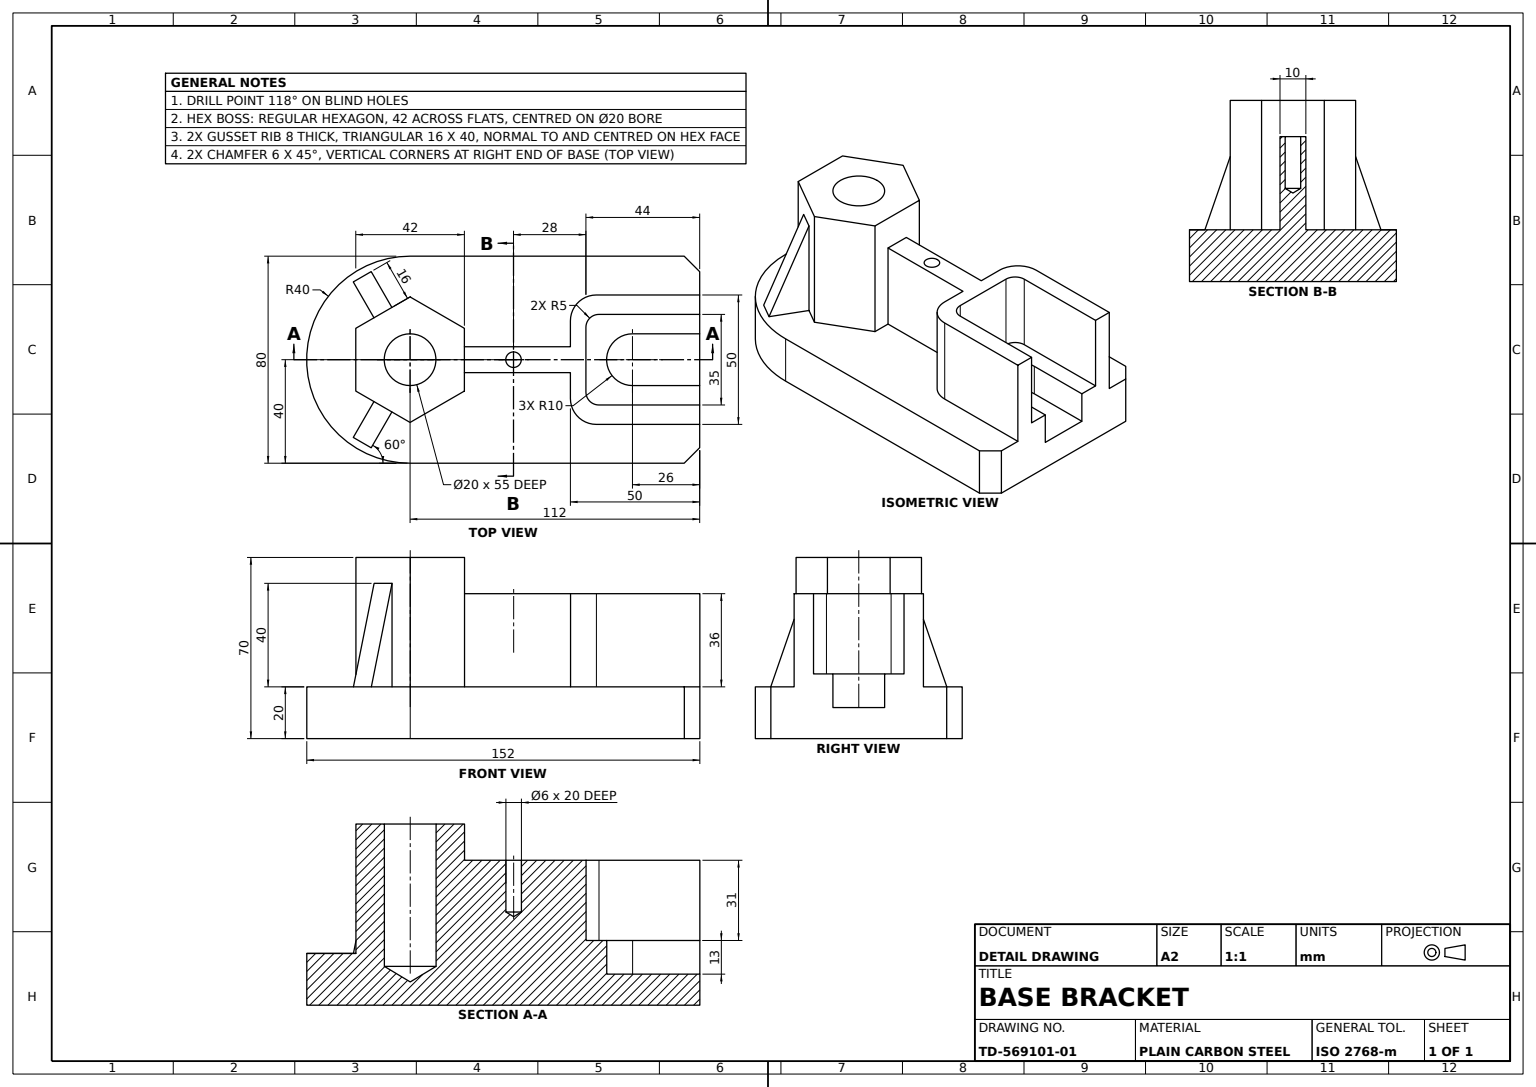
from build123d import *

# Parameters (mm, degrees)
BASE_PLATE_DEPTH        = 20
HEX_MOUNTING_BOSS_DEPTH = 50
GUSSET_RIB_1_SKETCH_W   = 8
GUSSET_RIB_1_SKETCH_H   = 40
GUSSET_RIB_1_DEPTH      = 16
RIB_1_TRIM_CUT_DEPTH    = 16
GUSSET_RIB_2_SKETCH_W   = 8
GUSSET_RIB_2_SKETCH_H   = 40
GUSSET_RIB_2_DEPTH      = 16
RIB_2_TRIM_CUT_DEPTH    = 16
BOSS_BORE_20_D          = 20
BOSS_BORE_20_DEPTH      = 55
BOSS_BORE_20_TIP        = 6.00860619
SHAFT_HOUSING_DEPTH     = 36
HOUSING_FILLET_R10_R    = 10
HOUSING_POCKET_DEPTH    = 31
HOUSING_SLOT_DEPTH      = 13
CROSS_HOLE_6_D          = 6
CROSS_HOLE_6_DEPTH      = 20
CROSS_HOLE_6_TIP        = 1.802581857


with BuildPart() as part:
    # Base Plate Sketch → Base Plate (new body)
    with BuildSketch(Plane(origin=(0, 0, 0), x_dir=(1, 0, 0), z_dir=(0, 1, 0))):
        with BuildLine():
            Line((0, 40), (106, 40))
            Line((106, 40), (112, 34))
            Line((112, 34), (112, -34))
            Line((112, -34), (106, -40))
            Line((106, -40), (0, -40))
            ThreePointArc((0, -40), (-40, 0), (0, 40))
        make_face()
    extrude(amount=BASE_PLATE_DEPTH)

    # Hex Boss Sketch → Hex Mounting Boss (add)
    with BuildSketch(Plane(origin=(0, 20, 0), x_dir=(1, 0, 0), z_dir=(0, 1, 0))):
        Polygon((0, 24.248711306), (-21, 12.124355653), (-21, -12.124355653), (0, -24.248711306), (21, -12.124355653), (21, 12.124355653), align=None)
    extrude(amount=HEX_MOUNTING_BOSS_DEPTH)

    # Gusset Rib 1 Sketch → Gusset Rib 1 (add)
    with BuildSketch(Plane(origin=(-10.5, 0, 18.186533479), x_dir=(0.8660254037844417, 0, 0.4999999999999949), z_dir=(-0.4999999999999949, 0, 0.8660254037844417))):
        with Locations((0, 40)):
            Rectangle(GUSSET_RIB_1_SKETCH_W, GUSSET_RIB_1_SKETCH_H)
    extrude(amount=GUSSET_RIB_1_DEPTH)

    # Rib 1 Trim Sketch → Rib 1 Trim Cut (cut)
    with BuildSketch(Plane(origin=(3.464101615, 0, 2), x_dir=(0.49999999999999495, 0, -0.8660254037844417), z_dir=(0.8660254037844417, 0, 0.49999999999999495))):
        Polygon((-21, 60), (-37, 20), (-37, 60), align=None)
    extrude(amount=-RIB_1_TRIM_CUT_DEPTH, mode=Mode.SUBTRACT)

    # Gusset Rib 2 Sketch → Gusset Rib 2 (add)
    with BuildSketch(Plane(origin=(-10.5, 0, -18.186533479), x_dir=(-0.8660254037844386, 0, 0.4999999999999999), z_dir=(-0.49999999999999994, 0, -0.8660254037844387))):
        with Locations((0, 40)):
            Rectangle(GUSSET_RIB_2_SKETCH_W, GUSSET_RIB_2_SKETCH_H)
    extrude(amount=GUSSET_RIB_2_DEPTH)

    # Rib 2 Trim Sketch → Rib 2 Trim Cut (cut)
    with BuildSketch(Plane(origin=(-3.464101615, 0, 2), x_dir=(0.5000000000000001, 0, 0.8660254037844386), z_dir=(-0.8660254037844386, 0, 0.5000000000000001))):
        Polygon((-21, 60), (-37, 20), (-37, 60), align=None)
    extrude(amount=-RIB_2_TRIM_CUT_DEPTH, mode=Mode.SUBTRACT)

    # Boss Bore Ø20
    with Locations(Plane(origin=(0, 70, 0), x_dir=(1, 0, 0), z_dir=(0, 1, 0))):
        with Locations((0, 0)):
            Hole(BOSS_BORE_20_D / 2, depth=BOSS_BORE_20_DEPTH)
            with Locations((0, 0, -(BOSS_BORE_20_DEPTH + BOSS_BORE_20_TIP / 2))):  # 118° drill point
                Cone(0, BOSS_BORE_20_D / 2, BOSS_BORE_20_TIP, mode=Mode.SUBTRACT)

    # Shaft Housing Sketch → Shaft Housing (add)
    with BuildSketch(Plane(origin=(0, 20, 0), x_dir=(1, 0, 0), z_dir=(0, 1, 0))):
        Polygon((112, 25), (62, 25), (62, 5), (21, 5), (21, -5), (62, -5), (62, -25), (112, -25), align=None)
    extrude(amount=SHAFT_HOUSING_DEPTH)

    # Housing Fillet R10
    housing_fillet_r10_edges = [part.edges().sort_by_distance(p)[0] for p in [
        (62, 38, -25),
        (62, 38, 25),
    ]]
    fillet(housing_fillet_r10_edges, radius=HOUSING_FILLET_R10_R)

    # Housing Pocket Sketch → Housing Pocket (cut)
    with BuildSketch(Plane(origin=(0, 56, 0), x_dir=(1, 0, 0), z_dir=(0, 1, 0))):
        with BuildLine():
            Line((112, 17.5), (73, 17.5))
            ThreePointArc((73, 17.5), (69.464466094, 16.035533906), (68, 12.5))
            Line((68, 12.5), (68, -12.5))
            ThreePointArc((68, -12.5), (69.464466094, -16.035533906), (73, -17.5))
            Line((73, -17.5), (112, -17.5))
            Line((112, -17.5), (112, 17.5))
        make_face()
    extrude(amount=-HOUSING_POCKET_DEPTH, mode=Mode.SUBTRACT)

    # Housing Slot Sketch → Housing Slot (cut)
    with BuildSketch(Plane(origin=(0, 25, 0), x_dir=(1, 0, 0), z_dir=(0, 1, 0))):
        with BuildLine():
            Line((86, 10), (112, 10))
            Line((112, 10), (112, -10))
            Line((112, -10), (86, -10))
            ThreePointArc((86, -10), (76, 0), (86, 10))
        make_face()
    extrude(amount=-HOUSING_SLOT_DEPTH, mode=Mode.SUBTRACT)

    # Cross Hole Ø6
    with Locations(Plane(origin=(0, 56, 0), x_dir=(1, 0, 0), z_dir=(0, 1, 0))):
        with Locations((40, 0)):
            Hole(CROSS_HOLE_6_D / 2, depth=CROSS_HOLE_6_DEPTH)
            with Locations((0, 0, -(CROSS_HOLE_6_DEPTH + CROSS_HOLE_6_TIP / 2))):  # 118° drill point
                Cone(0, CROSS_HOLE_6_D / 2, CROSS_HOLE_6_TIP, mode=Mode.SUBTRACT)


solid = part.part
